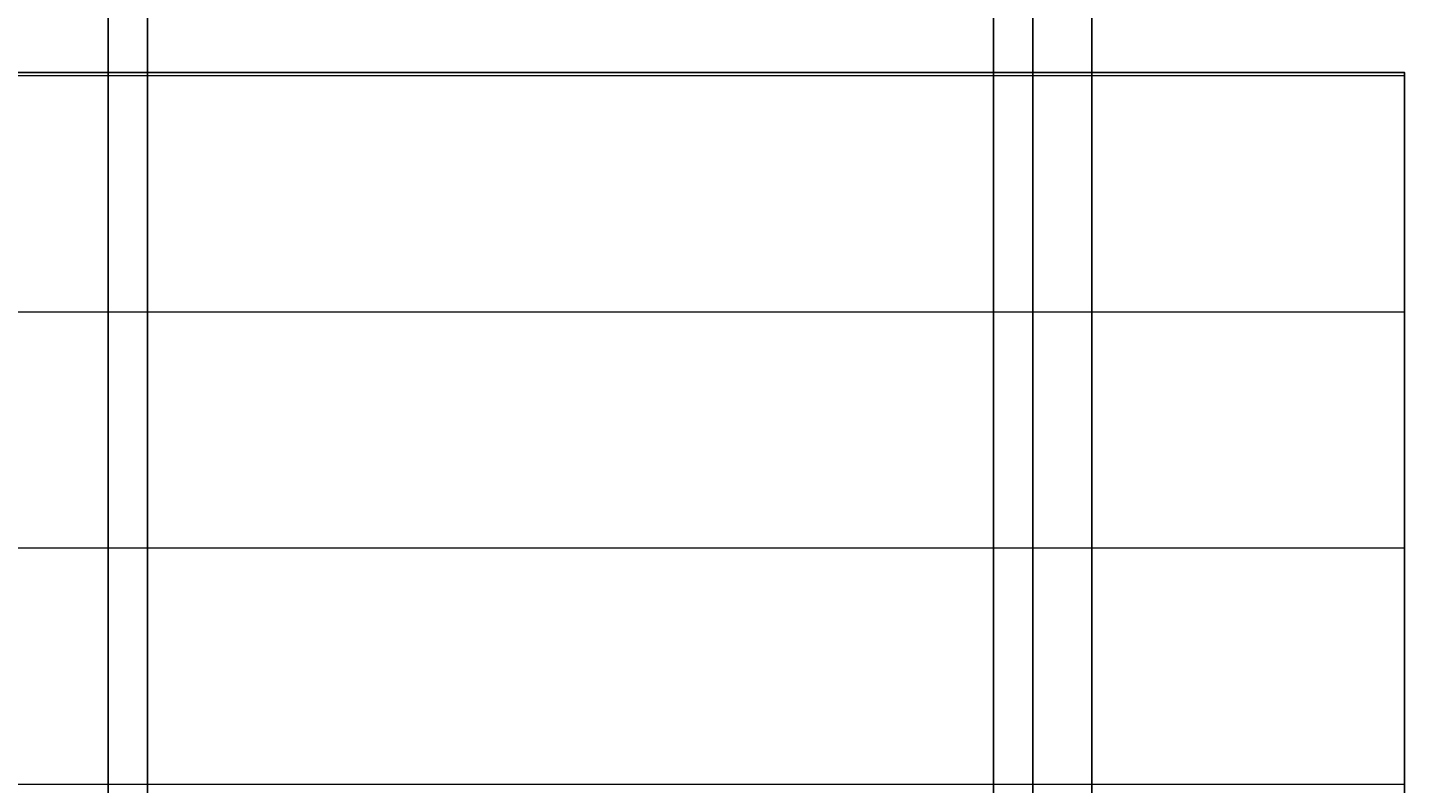
# Model space of a CAD drawing. Units: inches. Extents: x -6 to 289, y -8 to 323.
# Tile 33 of 107: x 209 to 244, y 30 to 49. Entities that reach past the tile are written whole.
import ezdxf

# ---------------------------------------------------------------- set-up
doc = ezdxf.new("R2010")
doc.units = ezdxf.units.IN
doc.header["$MEASUREMENT"] = 0
for name, color, linetype, lineweight in [('A-ANNO-DIMS', 2, 'Continuous', 18), ('A-DOOR', 3, 'Continuous', 25), ('A-ELEV-PATT', 8, 'Continuous', 13)]:
    doc.layers.add(name, color=color, linetype=linetype, lineweight=lineweight)
doc.styles.get("Standard").update_dxf_attribs({"font": 'arial.ttf'})
doc.dimstyles.get("Standard").update_dxf_attribs({"dimtxt": 0.18, "dimasz": 0.18, "dimexe": 0.18, "dimexo": 0.0625, "dimgap": 0.09, "dimtad": 0, "dimtih": 1, "dimtoh": 1, "dimdec": 4, "dimzin": 0, "dimdsep": 46, "dimtxsty": 'Standard', "dimcen": 0.09, "dimadec": 0, "dimazin": 0, "dimtfac": 1, "dimtdec": 4, "dimtofl": 0, "dimtmove": 0, "dimatfit": 3, "dimfxl": 1, "dimtolj": 1, "dimtzin": 0, "dimarcsym": 0})

# ---------------------------------------------------------------- blocks, each defined once
blk = doc.blocks.new('*D16')
at = {"layer": 'A-ANNO-DIMS', "color": 0, "lineweight": -2, "transparency": 16777216}
for p, q in [((9.943, 68.37), (9.943, -8.391)), ((272.973, 68.37), (272.973, -8.391)), ((10.123, -8.211), (140.993, -8.211)), ((272.793, -8.211), (141.923, -8.211))]:
    blk.add_line(p, q, dxfattribs=at)
at = {"layer": 'A-ANNO-DIMS', "color": 0, "transparency": 16777216}
for points in [[(10.123, -8.181), (10.123, -8.241), (9.943, -8.211)], [(272.793, -8.181), (272.793, -8.241), (272.973, -8.211)]]:
    blk.add_solid(points, dxfattribs=at)
at = {"layer": 'Defpoints', "color": 0, "transparency": 16777216}
for p in [(9.943, 68.432), (272.973, 68.432), (272.973, -8.211)]:
    blk.add_point(p, dxfattribs=at)
at = {"layer": 'A-ANNO-DIMS', "color": 0, "transparency": 16777216, "insert": (141.458, -8.211), "char_height": 0.18, "attachment_point": 5}
blk.add_mtext('\\A1;263.03', dxfattribs=at)
blk = doc.blocks.new('*D42')
at = {"layer": 'A-ANNO-DIMS', "color": 0, "lineweight": -2, "transparency": 16777216}
for p, q in [((190.792, 224.326), (190.792, -8.391)), ((211.292, 224.326), (211.292, -8.391)), ((190.972, -8.211), (200.716, -8.211)), ((211.112, -8.211), (201.368, -8.211))]:
    blk.add_line(p, q, dxfattribs=at)
at = {"layer": 'A-ANNO-DIMS', "color": 0, "transparency": 16777216}
for points in [[(190.972, -8.181), (190.972, -8.241), (190.792, -8.211)], [(211.112, -8.181), (211.112, -8.241), (211.292, -8.211)]]:
    blk.add_solid(points, dxfattribs=at)
at = {"layer": 'Defpoints', "color": 0, "transparency": 16777216}
for p in [(190.792, 224.389), (211.292, 224.389), (211.292, -8.211)]:
    blk.add_point(p, dxfattribs=at)
at = {"layer": 'A-ANNO-DIMS', "color": 0, "transparency": 16777216, "insert": (201.042, -8.211), "char_height": 0.18, "attachment_point": 5}
blk.add_mtext('\\A1;20.5', dxfattribs=at)
blk = doc.blocks.new('*D43')
at = {"layer": 'A-ANNO-DIMS', "color": 0, "lineweight": -2, "transparency": 16777216}
for p, q in [((211.292, 224.326), (211.292, -8.391)), ((212.292, 224.326), (212.292, -8.391)), ((211.472, -8.211), (211.669, -8.211)), ((212.112, -8.211), (211.915, -8.211))]:
    blk.add_line(p, q, dxfattribs=at)
at = {"layer": 'A-ANNO-DIMS', "color": 0, "transparency": 16777216}
for points in [[(211.472, -8.181), (211.472, -8.241), (211.292, -8.211)], [(212.112, -8.181), (212.112, -8.241), (212.292, -8.211)]]:
    blk.add_solid(points, dxfattribs=at)
at = {"layer": 'Defpoints', "color": 0, "transparency": 16777216}
for p in [(211.292, 224.389), (212.292, 224.389), (212.292, -8.211)]:
    blk.add_point(p, dxfattribs=at)
at = {"layer": 'A-ANNO-DIMS', "color": 0, "transparency": 16777216, "insert": (211.792, -8.211), "char_height": 0.18, "attachment_point": 5}
blk.add_mtext('\\A1;1', dxfattribs=at)
blk = doc.blocks.new('*D44')
at = {"layer": 'A-ANNO-DIMS', "color": 0, "lineweight": -2, "transparency": 16777216}
for p, q in [((212.292, 224.326), (212.292, -8.391)), ((233.792, 224.326), (233.792, -8.391)), ((212.472, -8.211), (222.716, -8.211)), ((233.612, -8.211), (223.368, -8.211))]:
    blk.add_line(p, q, dxfattribs=at)
at = {"layer": 'A-ANNO-DIMS', "color": 0, "transparency": 16777216}
for points in [[(212.472, -8.181), (212.472, -8.241), (212.292, -8.211)], [(233.612, -8.181), (233.612, -8.241), (233.792, -8.211)]]:
    blk.add_solid(points, dxfattribs=at)
at = {"layer": 'Defpoints', "color": 0, "transparency": 16777216}
for p in [(212.292, 224.389), (233.792, 224.389), (233.792, -8.211)]:
    blk.add_point(p, dxfattribs=at)
at = {"layer": 'A-ANNO-DIMS', "color": 0, "transparency": 16777216, "insert": (223.042, -8.211), "char_height": 0.18, "attachment_point": 5}
blk.add_mtext('\\A1;21.5', dxfattribs=at)
blk = doc.blocks.new('*D45')
at = {"layer": 'A-ANNO-DIMS', "color": 0, "lineweight": -2, "transparency": 16777216}
for p, q in [((234.792, 225.326), (234.792, -8.391)), ((233.792, 224.326), (233.792, -8.391)), ((233.972, -8.211), (234.169, -8.211)), ((234.612, -8.211), (234.415, -8.211))]:
    blk.add_line(p, q, dxfattribs=at)
at = {"layer": 'A-ANNO-DIMS', "color": 0, "transparency": 16777216}
for points in [[(233.972, -8.181), (233.972, -8.241), (233.792, -8.211)], [(234.612, -8.181), (234.612, -8.241), (234.792, -8.211)]]:
    blk.add_solid(points, dxfattribs=at)
at = {"layer": 'Defpoints', "color": 0, "transparency": 16777216}
for p in [(234.792, 225.389), (233.792, 224.389), (234.792, -8.211)]:
    blk.add_point(p, dxfattribs=at)
at = {"layer": 'A-ANNO-DIMS', "color": 0, "transparency": 16777216, "insert": (234.292, -8.211), "char_height": 0.18, "attachment_point": 5}
blk.add_mtext('\\A1;1', dxfattribs=at)
blk = doc.blocks.new('*D46')
at = {"layer": 'A-ANNO-DIMS', "color": 0, "lineweight": -2, "transparency": 16777216}
for p, q in [((236.292, 226.826), (236.292, -8.391)), ((234.792, 225.326), (234.792, -8.391)), ((234.972, -8.211), (235.296, -8.211)), ((236.112, -8.211), (235.788, -8.211))]:
    blk.add_line(p, q, dxfattribs=at)
at = {"layer": 'A-ANNO-DIMS', "color": 0, "transparency": 16777216}
for points in [[(234.972, -8.181), (234.972, -8.241), (234.792, -8.211)], [(236.112, -8.181), (236.112, -8.241), (236.292, -8.211)]]:
    blk.add_solid(points, dxfattribs=at)
at = {"layer": 'Defpoints', "color": 0, "transparency": 16777216}
for p in [(236.292, 226.889), (234.792, 225.389), (236.292, -8.211)]:
    blk.add_point(p, dxfattribs=at)
at = {"layer": 'A-ANNO-DIMS', "color": 0, "transparency": 16777216, "insert": (235.542, -8.211), "char_height": 0.18, "attachment_point": 5}
blk.add_mtext('\\A1;1.5', dxfattribs=at)

msp = doc.modelspace()

# ---------------------------------------------------------------- hatches: boundary and pattern name
at = {"layer": 'A-ELEV-PATT'}
h = msp.add_hatch(dxfattribs=at)
h.set_pattern_fill('_USER', color=256, scale=6, pattern_type=0)
h.set_pattern_definition([(0, (0, 0), (0, 6), [])])
h.paths.add_polyline_path([(184.1244, 48.0851), (124.008, 48.0851), (124.008, 10.2888), (184.1244, 10.2888)])
h.paths.add_polyline_path([(244.2408, 48.0851), (186.3604, 48.0851), (186.3604, 10.2888), (244.2408, 10.2888)])
h.paths.add_polyline_path([(208.2918, 114.2795), (190.7918, 114.2795), (190.7918, 71.2795), (208.2918, 71.2795)])
h.paths.add_polyline_path([(227.7918, 114.2795), (209.2918, 114.2795), (209.2918, 71.2795), (227.7918, 71.2795)])
h.paths.add_polyline_path([(211.2918, 224.3887), (190.7918, 224.3887), (190.7918, 162.3484), (211.2918, 162.3484)])
h.paths.add_polyline_path([(233.7918, 224.3887), (212.2918, 224.3887), (212.2918, 162.3484), (233.7918, 162.3484)])
h.paths.add_polyline_path([(166.3835, 224.154), (147.8835, 224.154), (147.8835, 181.154), (166.3835, 181.154)])
h.paths.add_polyline_path([(146.8835, 224.154), (129.3835, 224.154), (129.3835, 181.154), (146.8835, 181.154)])

# ---------------------------------------------------------------- linework, layer by layer
at = {"layer": 'A-DOOR'}
msp.add_lwpolyline([(124.008, 48.0851), (244.2408, 48.0851), (244.2408, 10.2888), (124.008, 10.2888)], close=True, dxfattribs=at)

# ---------------------------------------------------------------- dimensions: what is measured, and where the dimension line sits
at = {"layer": 'A-ANNO-DIMS'}
for base, p1, p2, override, picture, middle in [((236.2918, -8.2112), (234.7918, 225.3887), (236.2918, 226.8887), {"dimdec": 1, "dimlfac": 1, "dimrnd": 0, "dimzin": 0, "dimdsep": 46, "dimlunit": 2}, '*D46', (235.5418, -8.2112)), ((234.7918, -8.2112), (233.7918, 224.3887), (234.7918, 225.3887), {"dimdec": 0, "dimlfac": 1, "dimrnd": 0, "dimzin": 0, "dimdsep": 46, "dimlunit": 2}, '*D45', (234.2918, -8.2112)), ((211.2918, -8.2112), (190.7918, 224.3887), (211.2918, 224.3887), {"dimdec": 1, "dimlfac": 1, "dimrnd": 0, "dimzin": 0, "dimdsep": 46, "dimlunit": 2}, '*D42', (201.0418, -8.2112)), ((212.2918, -8.2112), (211.2918, 224.3887), (212.2918, 224.3887), {"dimdec": 0, "dimlfac": 1, "dimrnd": 0, "dimzin": 0, "dimdsep": 46, "dimlunit": 2}, '*D43', (211.7918, -8.2112)), ((233.7918, -8.2112), (212.2918, 224.3887), (233.7918, 224.3887), {"dimdec": 1, "dimlfac": 1, "dimrnd": 0, "dimzin": 0, "dimdsep": 46, "dimlunit": 2}, '*D44', (223.0418, -8.2112)), ((272.9733, -8.2112), (9.943, 68.4322), (272.9733, 68.4322), {"dimdec": 2, "dimlfac": 1, "dimrnd": 0, "dimzin": 0, "dimdsep": 46, "dimlunit": 2}, '*D16', (141.4581, -8.2112))]:
    dim = msp.add_linear_dim(base=base, p1=p1, p2=p2, dimstyle='Standard', override=override, dxfattribs=at)
    dim.commit()
    dim.dimension.update_dxf_attribs({"geometry": picture, "text_midpoint": middle})

doc.saveas('drawing.dxf')
